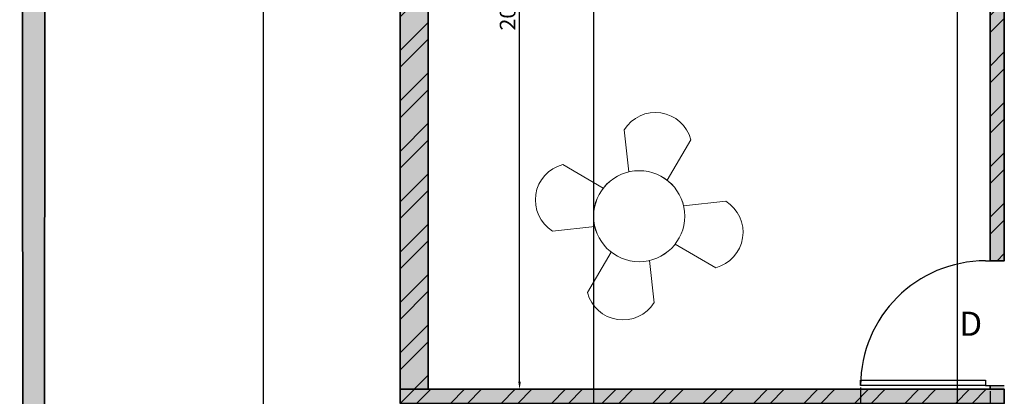
# Model space of a CAD drawing. Units: inches. Extents: x 1804 to 3296, y 909 to 2477.
# Tile 11 of 31: x 1804 to 2119, y 1542 to 1663. Entities that reach past the tile are written whole.
import ezdxf

# ---------------------------------------------------------------- set-up
doc = ezdxf.new("R2010")
doc.units = ezdxf.units.IN
for name, color, linetype, lineweight in [('A-ANNO-DIMS', 2, 'Continuous', 18), ('A-ANNO-TTLB', 156, 'Continuous', 35), ('A-WALL-PATT', 10, 'Continuous', 13), ('DOOR', 30, 'Continuous', 25), ('FUR', 100, 'Continuous', 18), ('TEXT', 190, 'Continuous', 18), ('WALL', 10, 'Continuous', 35)]:
    doc.layers.add(name, color=color, linetype=linetype, lineweight=lineweight)
doc.styles.get("Standard").update_dxf_attribs({"font": 'arial.ttf'})
doc.dimstyles.new('ISO-25', dxfattribs={"dimtxt": 5, "dimasz": 2.5, "dimexe": 1.25, "dimexo": 0.625, "dimtad": 1, "dimdec": 0, "dimlunit": 4, "dimtxsty": 'Standard', "dimcen": 2.5, "dimadec": 0, "dimazin": 0, "dimtfac": 1, "dimtdec": 0, "dimtmove": 0, "dimatfit": 3, "dimfxl": 1, "dimarcsym": 0})
pattern_1 = [(45, (0, 196.207), (-8.08223, 8.08223), []), (45, (5.388, 196.207), (-8.08223, 8.08223), [])]

# ---------------------------------------------------------------- blocks, each defined once
blk = doc.blocks.new('*U2')
for p, q in [((0, 0), (0, -6)), ((40, 0), (40, -6))]:
    blk.add_line(p, q)
blk.add_lwpolyline([(0, 0), (0, 40), (1.75, 40), (1.75, 0)], close=True)
blk.add_arc((0, 0), 40, 0, 90)
blk = doc.blocks.new('*U6')
for p, q in [((-4.25, 4.88), (-5.75, 18.4)), ((7.97, 2.19), (15.56, 15.17))]:
    blk.add_line(p, q)
blk.add_circle((-0.97, -9.34), 14.59)
blk.add_arc((4.21, 12.19), 11.73, 14.6829, 148.0797)
blk = doc.blocks.new('*U7')
at = {"layer": 'FUR', "transparency": 16777216}
blk.add_blockref('*U6', (1241.51, 881.82), dxfattribs=at)
for p, rotation in [((1231.21, 873.45), 89.99999999999999), ((1239.57, 863.15), 180), ((1249.88, 871.52), 269.9999999999999)]:
    blk.add_blockref('*U6', p, dxfattribs=dict(at, rotation=rotation))
blk = doc.blocks.new('*D9')
at = {"layer": 'A-ANNO-DIMS', "color": 0, "lineweight": -2, "transparency": 16777216}
for p, q in [((1935.21, 1793.38), (1965.1, 1793.38)), ((1963.85, 1546.88), (1963.85, 1790.88)), ((1935.21, 1544.38), (1965.1, 1544.38))]:
    blk.add_line(p, q, dxfattribs=at)
at = {"layer": 'A-ANNO-DIMS', "color": 0, "lineweight": 100, "transparency": 16777216}
for points in [[(1963.44, 1790.88), (1964.27, 1790.88), (1963.85, 1793.38)], [(1963.44, 1546.88), (1964.27, 1546.88), (1963.85, 1544.38)]]:
    blk.add_solid(points, dxfattribs=at)
at = {"layer": 'Defpoints', "color": 0, "lineweight": 100, "transparency": 16777216}
for p in [(1934.58, 1793.38), (1963.85, 1793.38), (1934.58, 1544.38)]:
    blk.add_point(p, dxfattribs=at)
at = {"layer": 'A-ANNO-DIMS', "color": 0, "transparency": 16777216, "insert": (1960.67, 1668.88), "char_height": 5, "attachment_point": 5, "rotation": 90}
blk.add_mtext('20\'-9"', dxfattribs=at)
blk = doc.blocks.new('*D52')
at = {"layer": 'A-ANNO-DIMS', "color": 0, "lineweight": -2, "transparency": 16777216}
for p, q in [((1924.96, 1830.04), (1880.63, 1830.04)), ((1881.88, 1065.27), (1881.88, 1827.54)), ((1924.96, 1062.77), (1880.63, 1062.77))]:
    blk.add_line(p, q, dxfattribs=at)
at = {"layer": 'A-ANNO-DIMS', "color": 0, "lineweight": 100, "transparency": 16777216}
for points in [[(1881.47, 1827.54), (1882.3, 1827.54), (1881.88, 1830.04)], [(1881.47, 1065.27), (1882.3, 1065.27), (1881.88, 1062.77)]]:
    blk.add_solid(points, dxfattribs=at)
at = {"layer": 'Defpoints', "color": 0, "lineweight": 100, "transparency": 16777216}
for p in [(1881.88, 1830.04), (1925.58, 1830.04), (1925.58, 1062.77)]:
    blk.add_point(p, dxfattribs=at)
at = {"layer": 'A-ANNO-DIMS', "color": 0, "transparency": 16777216, "insert": (1878.67, 1446.4), "char_height": 5, "attachment_point": 5, "rotation": 90}
blk.add_mtext('63\'-11 1/2"', dxfattribs=at)
blk = doc.blocks.new('*D60')
at = {"layer": 'A-ANNO-DIMS', "color": 0, "lineweight": -2, "transparency": 16777216}
for p, q in [((2073.08, 1544.95), (2073.08, 975.89)), ((2114.58, 1543.75), (2114.58, 975.89)), ((2112.08, 977.14), (2075.58, 977.14))]:
    blk.add_line(p, q, dxfattribs=at)
at = {"layer": 'A-ANNO-DIMS', "color": 0, "lineweight": 100, "transparency": 16777216}
for points in [[(2075.58, 977.56), (2075.58, 976.72), (2073.08, 977.14)], [(2112.08, 977.56), (2112.08, 976.72), (2114.58, 977.14)]]:
    blk.add_solid(points, dxfattribs=at)
at = {"layer": 'Defpoints', "color": 0, "lineweight": 100, "transparency": 16777216}
for p in [(2073.08, 1545.58), (2114.58, 1544.38), (2073.08, 977.14)]:
    blk.add_point(p, dxfattribs=at)
at = {"layer": 'A-ANNO-DIMS', "color": 0, "transparency": 16777216, "insert": (2093.83, 980.35), "char_height": 5, "attachment_point": 5}
blk.add_mtext('3\'-5 1/2"', dxfattribs=at)
blk = doc.blocks.new('*D62')
at = {"layer": 'A-ANNO-DIMS', "color": 0, "lineweight": -2, "transparency": 16777216}
for p, q in [((1987.63, 1501.57), (1987.63, 1874.99)), ((1990.13, 1873.74), (2101.57, 1873.74)), ((2104.07, 1501.57), (2104.07, 1874.99))]:
    blk.add_line(p, q, dxfattribs=at)
at = {"layer": 'A-ANNO-DIMS', "color": 0, "lineweight": 100, "transparency": 16777216}
for points in [[(1990.13, 1874.15), (1990.13, 1873.32), (1987.63, 1873.74)], [(2101.57, 1874.15), (2101.57, 1873.32), (2104.07, 1873.74)]]:
    blk.add_solid(points, dxfattribs=at)
at = {"layer": 'Defpoints', "color": 0, "lineweight": 100, "transparency": 16777216}
for p in [(2104.07, 1873.74), (1987.63, 1500.95), (2104.07, 1500.95)]:
    blk.add_point(p, dxfattribs=at)
at = {"layer": 'A-ANNO-DIMS', "color": 0, "transparency": 16777216, "insert": (2045.85, 1876.95), "char_height": 5, "attachment_point": 5}
blk.add_mtext('9\'-8 1/2"', dxfattribs=at)

msp = doc.modelspace()

# ---------------------------------------------------------------- hatches: boundary and pattern name
at = {"layer": 'A-ANNO-TTLB'}
h = msp.add_hatch(color=256, dxfattribs=at)
h.dxf.hatch_style = 1
h.paths.add_polyline_path([(3294.53, 2476.54), (1803.79, 2476.54), (1805.43, 909.47), (3296.17, 909.47)])
h.paths.add_polyline_path([(1811, 914.33), (1812.79, 2467.54), (3285.53, 2467.54), (3283.74, 914.33)], flags=16)
h.paths.add_polyline_path([(1925.58, 1062.77), (1925.58, 1138.07), (1925.58, 1539.88), (1925.58, 1793.38), (1925.58, 1830.04), (2325.54, 1830.04), (2325.54, 1793.38), (2325.54, 1586.42), (2325.54, 1138.07), (2325.54, 1062.77)], flags=0)
h.paths.add_polyline_path([(1997.22, 1029.4), (2008.85, 1037.96), (2008.85, 1020.84)], flags=0)
h.paths.add_polyline_path([(1934.58, 1138.07), (1934.58, 1147.07), (2078.77, 1147.07), (2078.77, 1138.07), (2060.94, 1138.07)], flags=0)
h.paths.add_polyline_path([(1944.35, 1138.07), (1944.35, 1147.07), (2056.05, 1147.07), (2056.05, 1138.07)], flags=0)
h.paths.add_polyline_path([(2222.24, 1037.96), (2233.87, 1029.4), (2222.24, 1020.84)], flags=0)
h.paths.add_polyline_path([(2061.94, 1139.07), (2061.94, 1146.07), (2077.77, 1146.07), (2077.77, 1139.07)], flags=0)
h.paths.add_polyline_path([(2149.58, 1138.07), (2149.58, 1269.44), (2158.58, 1269.44), (2158.58, 1326.69), (2149.58, 1326.69), (2149.58, 1340.94), (2139.6, 1340.94), (2139.6, 1434.25), (2149.58, 1434.25), (2149.58, 1447.36), (2158.58, 1447.36), (2158.58, 1423.87), (2158.58, 1408.06), (2198.46, 1408.06), (2198.46, 1412.56), (2282.65, 1412.56), (2282.65, 1465.94), (2316.54, 1465.94), (2316.54, 1590.92), (2192.86, 1590.92), (2192.86, 1595.3), (2291.17, 1595.3), (2291.17, 1590.92), (2316.54, 1590.92), (2316.54, 1784.38), (2300.24, 1784.38), (2300.24, 1757.47), (2268, 1757.47), (2268, 1681.04), (2180.87, 1681.04), (2180.87, 1757.47), (2148.63, 1757.47), (2148.63, 1784.38), (2119.08, 1784.38), (2119.08, 1585.58), (2114.58, 1585.58), (2114.58, 1784.38), (2064.11, 1784.38), (2046.28, 1784.38), (2046.28, 1760.38), (1958.58, 1760.38), (1958.58, 1664.38), (1934.58, 1664.38), (1934.58, 1784.38), (1934.58, 1793.38), (2046.28, 1793.38), (2064.11, 1793.38), (2119.08, 1793.38), (2230.78, 1793.38), (2230.78, 1784.38), (2268, 1784.38), (2300.24, 1784.38), (2316.54, 1784.38), (2316.54, 1590.92), (2316.54, 1373.73), (2316.54, 1138.07)], flags=0)
h.paths.add_polyline_path([(2209.19, 1166.63), (2209.19, 1175.63), (2158.58, 1175.63), (2209.19, 1223.63), (2209.19, 1231.63), (2183.88, 1231.63), (2183.88, 1301.66), (2242.59, 1301.66), (2242.59, 1326.69), (2316.54, 1326.69), (2272.59, 1271.63), (2272.59, 1223.63), (2316.54, 1175.63), (2272.59, 1175.63), (2272.59, 1166.63)], flags=0)
h.paths.add_polyline_path([(1947.77, 1345.22), (1947.77, 1457.48), (1991.2, 1457.48), (1991.2, 1451.7), (1991.2, 1352.18), (1991.2, 1345.22)], flags=0)
h.paths.add_polyline_path([(2209.19, 1271.63), (2262.59, 1271.63), (2262.59, 1311.85), (2272.59, 1301.66), (2272.59, 1271.63), (2269.92, 1269.63), (2270.59, 1269.63), (2270.59, 1225.63), (2211.19, 1225.63), (2211.19, 1269.63), (2211.86, 1269.63)], flags=0)
h.paths.add_polyline_path([(2000.34, 1378.21), (2000.34, 1429.71), (2025.22, 1429.71), (2025.22, 1378.21)], flags=0)
h.paths.add_polyline_path([(2001.34, 1379.21), (2001.34, 1428.71), (2024.22, 1428.71), (2024.22, 1379.21)], flags=0)
h.paths.add_polyline_path([(2012.34, 1390.21), (2012.34, 1417.71), (2013.22, 1417.71), (2013.22, 1390.21)], flags=0)
h.paths.add_polyline_path([(2237.56, 1331.19), (2237.56, 1340.18), (2238.62, 1340.18), (2238.62, 1386.84), (2241.04, 1386.84), (2242.06, 1386.84), (2242.06, 1408.06), (2316.54, 1331.19)], flags=0)
h.paths.add_polyline_path([(1953.73, 1464.35), (1953.73, 1498.59), (1981.74, 1498.59), (1981.74, 1464.35)], flags=0)
h.paths.add_polyline_path([(1987.63, 1462.08), (1987.63, 1500.95), (2104.07, 1500.95), (2104.07, 1462.08), (2099.27, 1462.08), (1993.6, 1462.08)], flags=0)
h.paths.add_polyline_path([(1956.06, 1481.47, -1), (1979.41, 1481.47, -1)], flags=0)
edge = h.paths.add_edge_path(flags=0)
edge.add_ellipse((2299.53, 1438.37), major_axis=(0.31, 21.36), ratio=0.670333, start_angle=0, end_angle=360)
h.paths.add_polyline_path([(2297.39, 1438.37, -1), (2301.67, 1438.37, -1)], flags=0)
h.paths.add_polyline_path([(2591.54, 1163.23), (2591.54, 1179.38), (2591.54, 1379.68), (2591.54, 1395.84), (2734.5, 1395.84), (2734.5, 1379.68), (2734.5, 1179.38), (2734.5, 1163.23)], flags=0)
h.paths.add_polyline_path([(2592.54, 1164.23), (2592.54, 1166.23), (2733.5, 1166.23), (2733.5, 1164.23)], flags=0)
h.paths.add_polyline_path([(2592.54, 1180.38), (2592.54, 1378.68), (2733.5, 1378.68), (2733.5, 1180.38)], flags=0)
h.paths.add_polyline_path([(2593.54, 1181.38), (2593.54, 1377.68), (2732.5, 1377.68), (2732.5, 1181.38)], flags=0)
h.paths.add_polyline_path([(2594.54, 1182.38), (2594.54, 1376.68), (2731.5, 1376.68), (2731.5, 1182.38)], flags=0)
h.paths.add_polyline_path([(1936.95, 1697.46), (1936.95, 1736.46), (1955.41, 1736.46), (1955.41, 1697.46)], flags=0)
h.paths.add_polyline_path([(1938.48, 1718.36), (1938.48, 1734.92), (1953.65, 1734.92), (1953.65, 1718.36)], flags=0)
h.paths.add_polyline_path([(1944.75, 1726.64, -1), (1947.37, 1726.64, -1)], flags=0)
h.paths.add_polyline_path([(2592.54, 1394.84), (2733.5, 1394.84), (2733.5, 1392.84), (2592.54, 1392.84)], flags=0)
h.paths.add_polyline_path([(1976.61, 1762.5), (1976.61, 1781.44), (2012.79, 1781.44), (2012.79, 1762.5)], flags=0)
h.paths.add_polyline_path([(1979.57, 1771.97, -1), (1991.39, 1771.97, -1)], flags=0)
h.paths.add_polyline_path([(1995.36, 1771.97, -1), (2007.18, 1771.97, -1)], flags=0)
h.paths.add_polyline_path([(2251.51, 1744.53), (2268, 1730.05), (2251.51, 1730.05)], flags=0)
h.paths.add_polyline_path([(2047.28, 1785.38), (2047.28, 1792.38), (2063.11, 1792.38), (2063.11, 1785.38)], flags=0)
h.paths.add_polyline_path([(2155.08, 1770.92, -1), (2174.42, 1770.92, -1)], flags=0)
h.paths.add_polyline_path([(2188.59, 1758.27), (2188.59, 1772.81), (2222.3, 1772.81), (2222.3, 1758.27)], flags=0)
h.paths.add_polyline_path([(2223.97, 1758.27), (2223.97, 1772.81), (2257.68, 1772.81), (2257.68, 1758.27)], flags=0)
h.paths.add_polyline_path([(2274.45, 1770.92, -1), (2293.8, 1770.92, -1)], flags=0)
h.paths.add_polyline_path([(2591.54, 1582.09), (2591.54, 1782.39), (2734.5, 1782.39), (2734.5, 1582.09)], flags=0)
h.paths.add_polyline_path([(2592.54, 1583.09), (2592.54, 1781.39), (2733.5, 1781.39), (2733.5, 1583.09)], flags=0)
h.paths.add_polyline_path([(2593.54, 1584.09), (2593.54, 1780.39), (2732.5, 1780.39), (2732.5, 1584.09)], flags=0)
h.paths.add_polyline_path([(2594.54, 1585.09), (2594.54, 1779.39), (2731.5, 1779.39), (2731.5, 1585.09)], flags=0)
h.paths.add_polyline_path([(1922.17, 1978.79), (1922.17, 2295.08), (1922.17, 2296.08), (2115.67, 2296.08), (2115.67, 2384.31), (2115.67, 2385.31), (2322.12, 2385.31), (2323.12, 2385.31), (2323.12, 1979.79), (2323.12, 1978.79), (1923.17, 1978.79)], flags=0)
h.paths.add_polyline_path([(1922.17, 1978.79), (1922.17, 2051.31), (1922.17, 2214.86), (1922.17, 2296.08), (2115.67, 2296.08), (2115.67, 2385.31), (2323.12, 2385.31), (2323.12, 2280.42), (2323.12, 1978.79), (2115.67, 1978.79)], flags=0)
h.paths.add_polyline_path([(1923.17, 1979.79), (1923.17, 2050.31), (2115.67, 2050.31), (2115.67, 2051.31), (1923.17, 2051.31), (1923.17, 2213.86), (1923.17, 2214.86), (1923.17, 2295.08), (1990.02, 2295.08), (1990.02, 2214.86), (1991.02, 2214.86), (1991.02, 2295.08), (2115.67, 2295.08), (2115.67, 1979.79), (2116.67, 1979.79), (2116.67, 2304.18), (2116.67, 2384.31), (2322.12, 2384.31), (2322.12, 2280.42), (2322.12, 1979.79), (2115.67, 1979.79)], flags=0)
h.paths.add_polyline_path([(2972.46, 1192.5), (2972.46, 1196.92), (2995.47, 1196.92), (2995.47, 1255.47), (2995.09, 1255.47), (2987.42, 1249.39), (2980.08, 1255.47), (2978.05, 1255.47), (2978.05, 1257.24), (2995.47, 1257.24), (2995.47, 1261.58), (3015.37, 1261.58), (3015.37, 1333.28), (3015.37, 1414.4), (3032.82, 1414.4), (3032.82, 1333.28), (3032.82, 1261.58), (3052.66, 1261.58), (3052.66, 1255.47), (3079.86, 1255.47), (3078.72, 1254.57), (3081.47, 1252.29), (3078.56, 1249.99), (3075.81, 1252.26), (3072.57, 1249.69), (3070.36, 1251.52), (3067.67, 1249.39), (3060.34, 1255.47), (3052.66, 1255.47), (3052.66, 1196.92), (3054.58, 1196.92), (3074, 1196.92), (3074, 1192.5), (3052.66, 1192.5), (2995.47, 1192.5)], flags=0)
h.paths.add_polyline_path([(2490.75, 1979.27), (2490.75, 1980.27), (2596.87, 1980.27), (2596.87, 2051.8), (2596.87, 2052.8), (2596.87, 2216.35), (2596.87, 2297.57), (2717.32, 2297.57), (2710.57, 2305.62), (2724.07, 2305.62), (2717.32, 2297.57), (2782.37, 2297.57), (2782.37, 2395.8), (3006.82, 2395.8), (3006.82, 1981.27), (3093.73, 1981.27), (3093.73, 1980.27), (3047.51, 1980.27), (3046.37, 1979.37), (3049.11, 1977.1), (3046.2, 1974.79), (3043.46, 1977.07), (3040.21, 1974.49), (3038, 1976.32), (3035.32, 1974.2), (3027.98, 1980.27), (2871.83, 1980.27), (2871.83, 1981.27), (2791.37, 1981.27), (2791.37, 2050.8), (2597.87, 2050.8), (2597.87, 1980.27), (2597.87, 1979.27), (2546.27, 1979.27), (2545.12, 1978.37), (2547.87, 1976.1), (2544.96, 1973.79), (2542.22, 1976.07), (2538.97, 1973.49), (2536.76, 1975.32), (2534.07, 1973.2), (2526.74, 1979.27)], flags=0)
h.paths.add_polyline_path([(2597.87, 2051.8), (2606.87, 2051.8), (2606.87, 2258.39), (2597.87, 2258.39), (2597.87, 2296.57), (2606.87, 2296.57), (2606.87, 2262.39), (2782.37, 2262.39), (2782.37, 2296.57), (2790.37, 2296.57), (2790.37, 2262.39), (2791.37, 2262.39), (2791.37, 2305.67), (2791.37, 2385.8), (2996.82, 2385.8), (2996.82, 2339.85), (3006.82, 2339.85), (3006.82, 2250.12), (2997.82, 2250.12), (2997.82, 1981.27), (2996.82, 1981.27), (2872.83, 1981.27), (2872.83, 1991.8), (2871.83, 1991.8), (2871.83, 2050.8), (2790.37, 2050.8), (2597.87, 2050.8)], flags=0)
h.paths.add_polyline_path([(2179.93, 2153.92), (2179.93, 2353.97), (2259.98, 2353.97), (2259.98, 2153.92)], flags=0)
h.paths.add_polyline_path([(2180.93, 2154.92), (2180.93, 2352.97), (2258.98, 2352.97), (2258.98, 2154.92)], flags=0)
h.paths.add_polyline_path([(2960.87, 1608.49), (2960.87, 1753.62), (3070.9, 1753.62), (3070.9, 1608.49)], flags=0)
h.paths.add_polyline_path([(2961.87, 1609.49), (2961.87, 1752.62), (3069.9, 1752.62), (3069.9, 1609.49)], flags=0)
h.paths.add_polyline_path([(2962.87, 1610.49), (2962.87, 1751.62), (3068.9, 1751.62), (3068.9, 1610.49)], flags=0)
h.paths.add_polyline_path([(2963.87, 1611.49), (2963.87, 1750.62), (3067.9, 1750.62), (3067.9, 1611.49)], flags=0)
h.paths.add_polyline_path([(2782.37, 2051.8), (2782.37, 2216.32), (2791.37, 2216.32), (2791.37, 2051.8), (2872.83, 2051.8), (2872.83, 2068.56), (2884.67, 2068.56), (2884.67, 2085.33), (2896.51, 2085.33), (2896.51, 2102.09), (2908.36, 2102.09), (2908.36, 2118.85), (2920.2, 2118.85), (2920.2, 2135.62), (2932.05, 2135.62), (2932.05, 2145.3), (2925.08, 2145.3), (2925.08, 2203.2), (2996.82, 2203.2), (2996.82, 2145.3), (2953.82, 2145.3), (2872.83, 2051.8), (2790.37, 2051.8)], flags=0)
h.paths.add_polyline_path([(2717.32, 2238.65), (2710.57, 2246.7), (2724.07, 2246.7)], flags=0)
h.paths.add_polyline_path([(2003.09, 1122.79), (2017.16, 1122.79), (2017.16, 1138.74), (2003.09, 1138.74)], flags=8)
h.paths.add_polyline_path([(2174.76, 1792.72), (2188.83, 1792.72), (2188.83, 1808.66), (2174.76, 1808.66)], flags=8)
h.paths.add_polyline_path([(1987.95, 1792.51), (2002.02, 1792.51), (2002.02, 1808.45), (1987.95, 1808.45)], flags=8)
h.paths.add_polyline_path([(2148.79, 1289.26), (2160.46, 1289.26), (2160.46, 1305.2), (2148.79, 1305.2)], flags=8)
h.paths.add_polyline_path([(2115.36, 1133.57), (2127.04, 1133.57), (2127.04, 1149.51), (2115.36, 1149.51)], flags=8)
h.paths.add_polyline_path([(2237.58, 1421.48), (2249.25, 1421.48), (2249.25, 1437.43), (2237.58, 1437.43)], flags=8)
h.paths.add_polyline_path([(2134.99, 1584.32), (2146.66, 1584.32), (2146.66, 1600.26), (2134.99, 1600.26)], flags=8)
h.paths.add_polyline_path([(2101.95, 1557.31), (2113.62, 1557.31), (2113.62, 1573.25), (2101.95, 1573.25)], flags=8)
h.paths.add_polyline_path([(2937.85, 1156.77), (3120.41, 1156.77), (3120.41, 1185.72), (2937.85, 1185.72)], flags=8)
h.paths.add_polyline_path([(2980.71, 1786.71), (3050.06, 1786.71), (3050.06, 1802.66), (2980.71, 1802.66)], flags=8)
h.paths.add_polyline_path([(2869.28, 1661.96), (2938.62, 1661.96), (2938.62, 1690.8), (2869.28, 1690.8)], flags=8)
h.paths.add_polyline_path([(3092.27, 1674.86), (3161.62, 1674.86), (3161.62, 1690.8), (3092.27, 1690.8)], flags=8)
h.paths.add_polyline_path([(2980.71, 1674.86), (3050.06, 1674.86), (3050.06, 1690.8), (2980.71, 1690.8)], flags=8)
h.paths.add_polyline_path([(2649.07, 1678.23), (2674.53, 1678.23), (2674.53, 1714.76), (2649.07, 1714.76)], flags=8)
h.paths.add_polyline_path([(2530.84, 1981.63), (2549.13, 1981.63), (2549.13, 1997.57), (2530.84, 1997.57)], flags=8)
h.paths.add_polyline_path([(3031.29, 1981.77), (3049.58, 1981.77), (3049.58, 1997.71), (3031.29, 1997.71)], flags=8)
h.paths.add_polyline_path([(2715.38, 1911.9), (2851.54, 1911.9), (2851.54, 1940.85), (2715.38, 1940.85)], flags=8)
h.paths.add_polyline_path([(2015.23, 1927.36), (2205.42, 1927.36), (2205.42, 1956.3), (2015.23, 1956.3)], flags=8)
h.paths.add_polyline_path([(2671.84, 2057.84), (2702.75, 2057.84), (2702.75, 2073.79), (2671.84, 2073.79)], flags=8)
h.paths.add_polyline_path([(2678.5, 2316.52), (2765.26, 2316.52), (2765.26, 2332.46), (2678.5, 2332.46)], flags=8)
h.paths.add_polyline_path([(2678.48, 2271.96), (2736.41, 2271.96), (2736.41, 2287.9), (2678.48, 2287.9)], flags=8)
h.paths.add_polyline_path([(2019.2, 972.79), (2243.21, 972.79), (2243.21, 1001.74), (2019.2, 1001.74)], flags=8)
h.paths.add_polyline_path([(2097.06, 1021.56), (2132.16, 1021.56), (2132.16, 1037.51), (2097.06, 1037.51)], flags=8)
h.paths.add_polyline_path([(2182.47, 1360.48), (2207.35, 1360.48), (2207.35, 1376.42), (2182.47, 1376.42)], flags=8)
h.paths.add_polyline_path([(2261.12, 1361.77), (2295.01, 1361.77), (2295.01, 1377.71), (2261.12, 1377.71)], flags=8)
h.paths.add_polyline_path([(2245.75, 1511.51), (2278.44, 1511.51), (2278.44, 1527.46), (2245.75, 1527.46)], flags=8)
h.paths.add_polyline_path([(1991.16, 1296.29), (2060.51, 1296.29), (2060.51, 1312.23), (1991.16, 1312.23)], flags=8)
h.paths.add_polyline_path([(2187, 1651.35), (2246.71, 1651.35), (2246.71, 1667.29), (2187, 1667.29)], flags=8)
h.paths.add_polyline_path([(1976.49, 1684.81), (2068.63, 1684.81), (2068.63, 1700.76), (1976.49, 1700.76)], flags=8)
at = {"layer": 'A-WALL-PATT'}
h = msp.add_hatch(color=256, dxfattribs=at)
h.dxf.hatch_style = 1
h.paths.add_polyline_path([(2119.08, 1544.38), (1925.58, 1544.38), (1925.58, 1539.88), (2119.08, 1539.88)])
h.paths.add_polyline_path([(2119.08, 1545.58), (2114.58, 1545.58), (2114.58, 1544.38), (2119.08, 1544.38)])
h.paths.add_polyline_path([(1965.87, 1658.79), (1965.87, 1679.09), (1955.57, 1679.09), (1955.57, 1658.79)], flags=9)
h.paths.add_polyline_path([(2293.18, 1677.29), (2293.18, 1697.58), (2282.88, 1697.58), (2282.88, 1677.29)], flags=9)
h.paths.add_polyline_path([(2271.13, 1545.23), (2287.53, 1545.23), (2287.53, 1555.53), (2271.13, 1555.53)], flags=9)
h.paths.add_polyline_path([(2303.26, 1488.52), (2303.26, 1508.82), (2292.95, 1508.82), (2292.95, 1488.52)], flags=9)
h.paths.add_polyline_path([(2271.13, 1393.15), (2287.53, 1393.15), (2287.53, 1403.45), (2271.13, 1403.45)], flags=9)
h.paths.add_polyline_path([(2306.48, 1361.45), (2306.48, 1377.86), (2296.18, 1377.86), (2296.18, 1361.45)], flags=9)
h.paths.add_polyline_path([(2174.54, 1361.45), (2174.54, 1377.86), (2164.23, 1377.86), (2164.23, 1361.45)], flags=9)
h.paths.add_polyline_path([(1968.21, 1333.34), (1968.21, 1353.64), (1957.91, 1353.64), (1957.91, 1333.34)], flags=9)
h.paths.add_polyline_path([(2003.09, 1122.79), (2017.16, 1122.79), (2017.16, 1138.74), (2003.09, 1138.74)], flags=9)
h.paths.add_polyline_path([(2174.76, 1792.72), (2188.83, 1792.72), (2188.83, 1808.66), (2174.76, 1808.66)], flags=9)
h.paths.add_polyline_path([(1987.95, 1792.51), (2002.02, 1792.51), (2002.02, 1808.45), (1987.95, 1808.45)], flags=9)
h.paths.add_polyline_path([(2148.79, 1289.26), (2160.46, 1289.26), (2160.46, 1305.2), (2148.79, 1305.2)], flags=9)
h.paths.add_polyline_path([(2115.36, 1133.57), (2127.04, 1133.57), (2127.04, 1149.51), (2115.36, 1149.51)], flags=9)
h.paths.add_polyline_path([(2237.58, 1421.48), (2249.25, 1421.48), (2249.25, 1437.43), (2237.58, 1437.43)], flags=9)
h.paths.add_polyline_path([(2134.99, 1584.32), (2146.66, 1584.32), (2146.66, 1600.26), (2134.99, 1600.26)], flags=9)
h.paths.add_polyline_path([(2101.95, 1557.31), (2113.62, 1557.31), (2113.62, 1573.25), (2101.95, 1573.25)], flags=9)
h.paths.add_polyline_path([(2937.85, 1156.77), (3120.41, 1156.77), (3120.41, 1185.72), (2937.85, 1185.72)], flags=9)
h.paths.add_polyline_path([(2980.71, 1786.71), (3050.06, 1786.71), (3050.06, 1802.66), (2980.71, 1802.66)], flags=9)
h.paths.add_polyline_path([(2869.28, 1661.96), (2938.62, 1661.96), (2938.62, 1690.8), (2869.28, 1690.8)], flags=9)
h.paths.add_polyline_path([(3092.27, 1674.86), (3161.62, 1674.86), (3161.62, 1690.8), (3092.27, 1690.8)], flags=9)
h.paths.add_polyline_path([(2980.71, 1674.86), (3050.06, 1674.86), (3050.06, 1690.8), (2980.71, 1690.8)], flags=9)
h.paths.add_polyline_path([(2649.07, 1678.23), (2674.53, 1678.23), (2674.53, 1714.76), (2649.07, 1714.76)], flags=9)
h.paths.add_polyline_path([(2530.84, 1981.63), (2549.13, 1981.63), (2549.13, 1997.57), (2530.84, 1997.57)], flags=9)
h.paths.add_polyline_path([(3031.29, 1981.77), (3049.58, 1981.77), (3049.58, 1997.71), (3031.29, 1997.71)], flags=9)
h.paths.add_polyline_path([(2715.38, 1911.9), (2851.54, 1911.9), (2851.54, 1940.85), (2715.38, 1940.85)], flags=9)
h.paths.add_polyline_path([(2015.23, 1927.36), (2205.42, 1927.36), (2205.42, 1956.3), (2015.23, 1956.3)], flags=9)
h.paths.add_polyline_path([(2671.84, 2057.84), (2702.75, 2057.84), (2702.75, 2073.79), (2671.84, 2073.79)], flags=9)
h.paths.add_polyline_path([(2678.5, 2316.52), (2765.26, 2316.52), (2765.26, 2332.46), (2678.5, 2332.46)], flags=9)
h.paths.add_polyline_path([(2678.48, 2271.96), (2736.41, 2271.96), (2736.41, 2287.9), (2678.48, 2287.9)], flags=9)
h.paths.add_polyline_path([(2019.2, 972.79), (2243.21, 972.79), (2243.21, 1001.74), (2019.2, 1001.74)], flags=9)
h.paths.add_polyline_path([(2097.06, 1021.56), (2132.16, 1021.56), (2132.16, 1037.51), (2097.06, 1037.51)], flags=9)
h.paths.add_polyline_path([(2182.47, 1360.48), (2207.35, 1360.48), (2207.35, 1376.42), (2182.47, 1376.42)], flags=9)
h.paths.add_polyline_path([(2261.12, 1361.77), (2295.01, 1361.77), (2295.01, 1377.71), (2261.12, 1377.71)], flags=9)
h.paths.add_polyline_path([(2245.75, 1511.51), (2278.44, 1511.51), (2278.44, 1527.46), (2245.75, 1527.46)], flags=9)
h.paths.add_polyline_path([(1991.16, 1296.29), (2060.51, 1296.29), (2060.51, 1312.23), (1991.16, 1312.23)], flags=9)
h.paths.add_polyline_path([(2187, 1651.35), (2246.71, 1651.35), (2246.71, 1667.29), (2187, 1667.29)], flags=9)
h.paths.add_polyline_path([(1976.49, 1684.81), (2068.63, 1684.81), (2068.63, 1700.76), (1976.49, 1700.76)], flags=9)
h = msp.add_hatch(color=256, dxfattribs=at)
h.dxf.hatch_style = 1
h.paths.add_polyline_path([(2149.58, 1147.07), (2141.21, 1147.07), (2141.21, 1144.07), (2141.21, 1138.07), (2149.58, 1138.07)])
h.paths.add_polyline_path([(2101.21, 1144.07, -0.01877), (2101.32, 1147.07), (2078.77, 1147.07), (2078.77, 1138.07), (2101.21, 1138.07)])
h.paths.add_polyline_path([(2060.94, 1147.07), (2056.05, 1147.07), (2056.05, 1138.07), (2060.94, 1138.07)])
h.paths.add_polyline_path([(1944.35, 1147.07), (1934.58, 1147.07), (1934.58, 1138.07), (1944.35, 1138.07)])
h.paths.add_polyline_path([(2158.58, 1269.44), (2149.58, 1269.44), (2149.58, 1138.07), (2158.58, 1138.07)])
h.paths.add_polyline_path([(2003.09, 1122.79), (2017.16, 1122.79), (2017.16, 1138.74), (2003.09, 1138.74)], flags=9)
h.paths.add_polyline_path([(2174.76, 1792.72), (2188.83, 1792.72), (2188.83, 1808.66), (2174.76, 1808.66)], flags=9)
h.paths.add_polyline_path([(1987.95, 1792.51), (2002.02, 1792.51), (2002.02, 1808.45), (1987.95, 1808.45)], flags=9)
h.paths.add_polyline_path([(2148.79, 1289.26), (2160.46, 1289.26), (2160.46, 1305.2), (2148.79, 1305.2)], flags=9)
h.paths.add_polyline_path([(2115.36, 1133.57), (2127.04, 1133.57), (2127.04, 1149.51), (2115.36, 1149.51)], flags=9)
h.paths.add_polyline_path([(2237.58, 1421.48), (2249.25, 1421.48), (2249.25, 1437.43), (2237.58, 1437.43)], flags=9)
h.paths.add_polyline_path([(2134.99, 1584.32), (2146.66, 1584.32), (2146.66, 1600.26), (2134.99, 1600.26)], flags=9)
h.paths.add_polyline_path([(2101.95, 1557.31), (2113.62, 1557.31), (2113.62, 1573.25), (2101.95, 1573.25)], flags=9)
h.paths.add_polyline_path([(2937.85, 1156.77), (3120.41, 1156.77), (3120.41, 1185.72), (2937.85, 1185.72)], flags=9)
h.paths.add_polyline_path([(2980.71, 1786.71), (3050.06, 1786.71), (3050.06, 1802.66), (2980.71, 1802.66)], flags=9)
h.paths.add_polyline_path([(2869.28, 1661.96), (2938.62, 1661.96), (2938.62, 1690.8), (2869.28, 1690.8)], flags=9)
h.paths.add_polyline_path([(3092.27, 1674.86), (3161.62, 1674.86), (3161.62, 1690.8), (3092.27, 1690.8)], flags=9)
h.paths.add_polyline_path([(2980.71, 1674.86), (3050.06, 1674.86), (3050.06, 1690.8), (2980.71, 1690.8)], flags=9)
h.paths.add_polyline_path([(2649.07, 1678.23), (2674.53, 1678.23), (2674.53, 1714.76), (2649.07, 1714.76)], flags=9)
h.paths.add_polyline_path([(2530.84, 1981.63), (2549.13, 1981.63), (2549.13, 1997.57), (2530.84, 1997.57)], flags=9)
h.paths.add_polyline_path([(3031.29, 1981.77), (3049.58, 1981.77), (3049.58, 1997.71), (3031.29, 1997.71)], flags=9)
h.paths.add_polyline_path([(2715.38, 1911.9), (2851.54, 1911.9), (2851.54, 1940.85), (2715.38, 1940.85)], flags=9)
h.paths.add_polyline_path([(2015.23, 1927.36), (2205.42, 1927.36), (2205.42, 1956.3), (2015.23, 1956.3)], flags=9)
h.paths.add_polyline_path([(2671.84, 2057.84), (2702.75, 2057.84), (2702.75, 2073.79), (2671.84, 2073.79)], flags=9)
h.paths.add_polyline_path([(2678.5, 2316.52), (2765.26, 2316.52), (2765.26, 2332.46), (2678.5, 2332.46)], flags=9)
h.paths.add_polyline_path([(2678.48, 2271.96), (2736.41, 2271.96), (2736.41, 2287.9), (2678.48, 2287.9)], flags=9)
h.paths.add_polyline_path([(2019.2, 972.79), (2243.21, 972.79), (2243.21, 1001.74), (2019.2, 1001.74)], flags=9)
h.paths.add_polyline_path([(2097.06, 1021.56), (2132.16, 1021.56), (2132.16, 1037.51), (2097.06, 1037.51)], flags=9)
h.paths.add_polyline_path([(2182.47, 1360.48), (2207.35, 1360.48), (2207.35, 1376.42), (2182.47, 1376.42)], flags=9)
h.paths.add_polyline_path([(2261.12, 1361.77), (2295.01, 1361.77), (2295.01, 1377.71), (2261.12, 1377.71)], flags=9)
h.paths.add_polyline_path([(2245.75, 1511.51), (2278.44, 1511.51), (2278.44, 1527.46), (2245.75, 1527.46)], flags=9)
h.paths.add_polyline_path([(1991.16, 1296.29), (2060.51, 1296.29), (2060.51, 1312.23), (1991.16, 1312.23)], flags=9)
h.paths.add_polyline_path([(2187, 1651.35), (2246.71, 1651.35), (2246.71, 1667.29), (2187, 1667.29)], flags=9)
h.paths.add_polyline_path([(1976.49, 1684.81), (2068.63, 1684.81), (2068.63, 1700.76), (1976.49, 1700.76)], flags=9)
h = msp.add_hatch(color=256, dxfattribs=at)
h.dxf.hatch_style = 1
h.paths.add_polyline_path([(2158.58, 1275.49), (2155.29, 1275.49), (2149.58, 1275.49), (2149.58, 1269.44), (2158.58, 1269.44)])
h.paths.add_polyline_path([(2158.58, 1326.69), (2149.58, 1326.69), (2149.58, 1319.33), (2155.29, 1319.33), (2158.58, 1319.33)])
h.paths.add_polyline_path([(2158.58, 1402.2), (2158.58, 1423.87), (2158.58, 1447.36), (2149.58, 1447.36), (2149.58, 1423.87), (2149.58, 1340.94), (2149.58, 1326.69), (2158.58, 1326.69), (2158.58, 1354.23)])
h.paths.add_polyline_path([(1965.87, 1658.79), (1965.87, 1679.09), (1955.57, 1679.09), (1955.57, 1658.79)], flags=9)
h.paths.add_polyline_path([(2293.18, 1677.29), (2293.18, 1697.58), (2282.88, 1697.58), (2282.88, 1677.29)], flags=9)
h.paths.add_polyline_path([(2271.13, 1545.23), (2287.53, 1545.23), (2287.53, 1555.53), (2271.13, 1555.53)], flags=9)
h.paths.add_polyline_path([(2303.26, 1488.52), (2303.26, 1508.82), (2292.95, 1508.82), (2292.95, 1488.52)], flags=9)
h.paths.add_polyline_path([(2271.13, 1393.15), (2287.53, 1393.15), (2287.53, 1403.45), (2271.13, 1403.45)], flags=9)
h.paths.add_polyline_path([(2306.48, 1361.45), (2306.48, 1377.86), (2296.18, 1377.86), (2296.18, 1361.45)], flags=9)
h.paths.add_polyline_path([(2189.9, 1340.62), (2206.31, 1340.62), (2206.31, 1350.92), (2189.9, 1350.92)], flags=9)
h.paths.add_polyline_path([(2174.54, 1361.45), (2174.54, 1377.86), (2164.23, 1377.86), (2164.23, 1361.45)], flags=9)
h.paths.add_polyline_path([(2304.24, 1240.8), (2304.24, 1261.09), (2293.94, 1261.09), (2293.94, 1240.8)], flags=9)
h.paths.add_polyline_path([(2227.19, 1188.73), (2247.49, 1188.73), (2247.49, 1199.03), (2227.19, 1199.03)], flags=9)
h.paths.add_polyline_path([(2181.93, 1144.21), (2181.93, 1160.62), (2171.63, 1160.62), (2171.63, 1144.21)], flags=9)
h.paths.add_polyline_path([(1968.21, 1333.34), (1968.21, 1353.64), (1957.91, 1353.64), (1957.91, 1333.34)], flags=9)
h.paths.add_polyline_path([(2029.78, 1203.53), (2053.95, 1203.53), (2053.95, 1213.83), (2029.78, 1213.83)], flags=9)
h.paths.add_polyline_path([(2576.51, 1671.88), (2576.51, 1692.17), (2566.21, 1692.17), (2566.21, 1671.88)], flags=9)
h.paths.add_polyline_path([(2566.99, 1269.67), (2566.99, 1289.96), (2556.68, 1289.96), (2556.68, 1269.67)], flags=9)
h.paths.add_polyline_path([(2581.85, 1269.17), (2581.85, 1289.46), (2571.54, 1289.46), (2571.54, 1269.17)], flags=9)
h.paths.add_polyline_path([(2650.71, 1409.75), (2674.89, 1409.75), (2674.89, 1420.05), (2650.71, 1420.05)], flags=9)
h.paths.add_polyline_path([(2003.09, 1122.79), (2017.16, 1122.79), (2017.16, 1138.74), (2003.09, 1138.74)], flags=9)
h.paths.add_polyline_path([(2174.76, 1792.72), (2188.83, 1792.72), (2188.83, 1808.66), (2174.76, 1808.66)], flags=9)
h.paths.add_polyline_path([(1987.95, 1792.51), (2002.02, 1792.51), (2002.02, 1808.45), (1987.95, 1808.45)], flags=9)
h.paths.add_polyline_path([(2148.79, 1289.26), (2160.46, 1289.26), (2160.46, 1305.2), (2148.79, 1305.2)], flags=9)
h.paths.add_polyline_path([(2115.36, 1133.57), (2127.04, 1133.57), (2127.04, 1149.51), (2115.36, 1149.51)], flags=9)
h.paths.add_polyline_path([(2237.58, 1421.48), (2249.25, 1421.48), (2249.25, 1437.43), (2237.58, 1437.43)], flags=9)
h.paths.add_polyline_path([(2134.99, 1584.32), (2146.66, 1584.32), (2146.66, 1600.26), (2134.99, 1600.26)], flags=9)
h.paths.add_polyline_path([(2101.95, 1557.31), (2113.62, 1557.31), (2113.62, 1573.25), (2101.95, 1573.25)], flags=9)
h.paths.add_polyline_path([(2937.85, 1156.77), (3120.41, 1156.77), (3120.41, 1185.72), (2937.85, 1185.72)], flags=9)
h.paths.add_polyline_path([(2980.71, 1786.71), (3050.06, 1786.71), (3050.06, 1802.66), (2980.71, 1802.66)], flags=9)
h.paths.add_polyline_path([(2869.28, 1661.96), (2938.62, 1661.96), (2938.62, 1690.8), (2869.28, 1690.8)], flags=9)
h.paths.add_polyline_path([(3092.27, 1674.86), (3161.62, 1674.86), (3161.62, 1690.8), (3092.27, 1690.8)], flags=9)
h.paths.add_polyline_path([(2980.71, 1674.86), (3050.06, 1674.86), (3050.06, 1690.8), (2980.71, 1690.8)], flags=9)
h.paths.add_polyline_path([(2649.07, 1678.23), (2674.53, 1678.23), (2674.53, 1714.76), (2649.07, 1714.76)], flags=9)
h.paths.add_polyline_path([(2530.84, 1981.63), (2549.13, 1981.63), (2549.13, 1997.57), (2530.84, 1997.57)], flags=9)
h.paths.add_polyline_path([(3031.29, 1981.77), (3049.58, 1981.77), (3049.58, 1997.71), (3031.29, 1997.71)], flags=9)
h.paths.add_polyline_path([(2715.38, 1911.9), (2851.54, 1911.9), (2851.54, 1940.85), (2715.38, 1940.85)], flags=9)
h.paths.add_polyline_path([(2015.23, 1927.36), (2205.42, 1927.36), (2205.42, 1956.3), (2015.23, 1956.3)], flags=9)
h.paths.add_polyline_path([(2671.84, 2057.84), (2702.75, 2057.84), (2702.75, 2073.79), (2671.84, 2073.79)], flags=9)
h.paths.add_polyline_path([(2678.5, 2316.52), (2765.26, 2316.52), (2765.26, 2332.46), (2678.5, 2332.46)], flags=9)
h.paths.add_polyline_path([(2678.48, 2271.96), (2736.41, 2271.96), (2736.41, 2287.9), (2678.48, 2287.9)], flags=9)
h.paths.add_polyline_path([(2019.2, 972.79), (2243.21, 972.79), (2243.21, 1001.74), (2019.2, 1001.74)], flags=9)
h.paths.add_polyline_path([(2097.06, 1021.56), (2132.16, 1021.56), (2132.16, 1037.51), (2097.06, 1037.51)], flags=9)
h.paths.add_polyline_path([(2182.47, 1360.48), (2207.35, 1360.48), (2207.35, 1376.42), (2182.47, 1376.42)], flags=9)
h.paths.add_polyline_path([(2261.12, 1361.77), (2295.01, 1361.77), (2295.01, 1377.71), (2261.12, 1377.71)], flags=9)
h.paths.add_polyline_path([(2245.75, 1511.51), (2278.44, 1511.51), (2278.44, 1527.46), (2245.75, 1527.46)], flags=9)
h.paths.add_polyline_path([(1991.16, 1296.29), (2060.51, 1296.29), (2060.51, 1312.23), (1991.16, 1312.23)], flags=9)
h.paths.add_polyline_path([(2187, 1651.35), (2246.71, 1651.35), (2246.71, 1667.29), (2187, 1667.29)], flags=9)
h.paths.add_polyline_path([(1976.49, 1684.81), (2068.63, 1684.81), (2068.63, 1700.76), (1976.49, 1700.76)], flags=9)
h = msp.add_hatch(dxfattribs=at)
h.set_pattern_fill('ANSI32', color=256, scale=1.2)
h.set_pattern_definition(pattern_1)
h.paths.add_polyline_path([(1934.58, 1784.38), (1934.58, 1793.38), (1925.58, 1793.38), (1925.58, 1539.88), (2119.08, 1539.88), (2119.08, 1545.58), (2114.58, 1545.58), (2114.58, 1544.38), (1934.58, 1544.38)])
h.paths.add_polyline_path([(2114.58, 1793.38), (2064.11, 1793.38), (2064.11, 1784.38), (2114.58, 1784.38)], flags=17)
h.paths.add_polyline_path([(2325.54, 1793.38), (2230.78, 1793.38), (2230.78, 1784.38), (2268, 1784.38), (2300.24, 1784.38), (2316.54, 1784.38), (2316.54, 1590.92), (2316.54, 1586.42), (2325.54, 1586.42)])
h.paths.add_polyline_path([(1944.35, 1147.07), (1934.58, 1147.07), (1934.58, 1138.07), (1944.35, 1138.07)])
h.paths.add_polyline_path([(2101.21, 1144.07, -0.01877), (2101.32, 1147.07), (2078.77, 1147.07), (2078.77, 1138.07), (2101.21, 1138.07)])
h.paths.add_polyline_path([(1934.58, 1539.88), (1925.58, 1539.88), (1925.58, 1138.07), (1934.58, 1138.07), (1934.58, 1147.07)])
h.paths.add_polyline_path([(2325.54, 1586.42), (2316.54, 1586.42), (2316.54, 1373.73), (2316.54, 1138.07), (2325.54, 1138.07), (2325.54, 1228.97)])
h.paths.add_polyline_path([(2158.58, 1423.87), (2158.58, 1447.36), (2149.58, 1447.36), (2149.58, 1423.87), (2149.58, 1340.94), (2149.58, 1326.69), (2158.58, 1326.69), (2158.58, 1354.23), (2158.58, 1402.2)])
h.paths.add_polyline_path([(2316.54, 1412.56), (2282.65, 1412.56), (2273.09, 1412.56), (2273.09, 1408.06), (2316.54, 1408.06)])
h.paths.add_polyline_path([(2273.09, 1412.56), (2242.06, 1412.56), (2242.06, 1408.06), (2273.09, 1408.06)])
h.paths.add_polyline_path([(2237.56, 1412.56), (2198.46, 1412.56), (2198.46, 1408.06), (2237.56, 1408.06)])
h.paths.add_polyline_path([(2242.06, 1408.06), (2237.56, 1408.06), (2237.56, 1386.84), (2242.06, 1386.84)])
h.paths.add_polyline_path([(2242.06, 1412.56), (2237.56, 1412.56), (2237.56, 1408.06), (2242.06, 1408.06)])
h.paths.add_polyline_path([(2158.58, 1269.44), (2149.58, 1269.44), (2149.58, 1138.07), (2158.58, 1138.07)])
h.paths.add_polyline_path([(2149.58, 1147.07), (2141.21, 1147.07), (2141.21, 1144.07), (2141.21, 1138.07), (2149.58, 1138.07)])
h.paths.add_polyline_path([(2272.59, 1175.63), (2209.19, 1175.63), (2209.19, 1166.63), (2272.59, 1166.63)])
h.paths.add_polyline_path([(2237.56, 1446.21), (2242.06, 1446.21), (2242.06, 1586.42), (2237.56, 1586.42)])
h.paths.add_polyline_path([(2242.06, 1414.58), (2237.56, 1414.58), (2237.56, 1412.56), (2242.06, 1412.56)])
h = msp.add_hatch(color=256, dxfattribs=at)
h.dxf.hatch_style = 1
h.paths.add_polyline_path([(1934.58, 1793.38), (1925.58, 1793.38), (1925.58, 1544.38), (1934.58, 1544.38)])
h.paths.add_polyline_path([(1934.58, 1539.88), (1925.58, 1539.88), (1925.58, 1138.07), (1934.58, 1138.07)])
h = msp.add_hatch(color=256, dxfattribs=at)
h.dxf.hatch_style = 1
h.paths.add_polyline_path([(2114.58, 1793.38), (2064.11, 1793.38), (2064.11, 1784.38), (2114.58, 1784.38)])
h.paths.add_polyline_path([(2119.08, 1793.38), (2114.58, 1793.38), (2114.58, 1585.58), (2119.08, 1585.58)])
h.paths.add_polyline_path([(2325.54, 1793.38), (2230.78, 1793.38), (2230.78, 1784.38), (2268, 1784.38), (2316.54, 1784.38), (2316.54, 1590.92), (2316.54, 1586.42), (2325.54, 1586.42)])
h.paths.add_polyline_path([(2316.54, 1331.19), (2158.58, 1331.19), (2158.58, 1326.69), (2316.54, 1326.69)])
h.paths.add_polyline_path([(2242.06, 1408.06), (2237.56, 1408.06), (2237.56, 1386.84), (2242.06, 1386.84)])
h.paths.add_polyline_path([(2242.06, 1412.56), (2237.56, 1412.56), (2237.56, 1408.06), (2242.06, 1408.06)])
h.paths.add_polyline_path([(2237.56, 1412.56), (2198.46, 1412.56), (2198.46, 1408.06), (2237.56, 1408.06)])
h.paths.add_polyline_path([(2273.09, 1412.56), (2242.06, 1412.56), (2242.06, 1408.06), (2273.09, 1408.06)])
h.paths.add_polyline_path([(2316.54, 1412.56), (2282.65, 1412.56), (2273.09, 1412.56), (2273.09, 1408.06), (2316.54, 1408.06)])
h.paths.add_polyline_path([(2325.54, 1586.42), (2316.54, 1586.42), (2316.54, 1373.73), (2316.54, 1138.07), (2325.54, 1138.07), (2325.54, 1228.97)])
h.paths.add_polyline_path([(2272.59, 1175.63), (2209.19, 1175.63), (2209.19, 1166.63), (2272.59, 1166.63)])
h = msp.add_hatch(dxfattribs=at)
h.set_pattern_fill('ANSI32', color=256, scale=1.2)
h.set_pattern_definition(pattern_1)
h.paths.add_polyline_path([(2114.58, 1585.58), (2119.08, 1585.58), (2119.08, 1793.38), (2114.58, 1793.38)])

# ---------------------------------------------------------------- linework, layer by layer
at = {"layer": 'A-ANNO-TTLB'}
for points in [[(1803.79, 2476.54), (3294.53, 2476.54), (3296.17, 909.47), (1805.43, 909.47)], [(1812.79, 2467.54), (3285.53, 2467.54), (3283.74, 914.33), (1811, 914.33)]]:
    msp.add_lwpolyline(points, close=True, dxfattribs=at)
at = {"layer": 'WALL'}
for p, q in [((1925.58, 1539.88), (1925.58, 1793.38)), ((1934.58, 1544.38), (1934.58, 1784.38)), ((2114.58, 1784.38), (2114.58, 1585.58)), ((2114.58, 1545.58), (2114.58, 1544.38)), ((2114.58, 1544.38), (1934.58, 1544.38))]:
    msp.add_line(p, q, dxfattribs=at)
for points in [[(1925.58, 1544.38), (1934.58, 1544.38), (1934.58, 1793.38), (1925.58, 1793.38)], [(2114.58, 1585.58), (2119.08, 1585.58), (2119.08, 1793.38), (2114.58, 1793.38)], [(1925.58, 1539.88), (2119.08, 1539.88), (2119.08, 1544.38), (1925.58, 1544.38)]]:
    msp.add_lwpolyline(points, close=True, dxfattribs=at)

# ---------------------------------------------------------------- block references
at = {"layer": 'DOOR', "rotation": 90}
msp.add_blockref('*U2', (2113.08, 1545.58), dxfattribs=at)
at = {"layer": 'FUR'}
msp.add_blockref('*U7', (761.62, 727.41), dxfattribs=at)

# ---------------------------------------------------------------- texts
at = {"layer": 'TEXT', "insert": (2104.72, 1569.27), "char_height": 7.74, "attachment_point": 1}
msp.add_mtext_dynamic_manual_height_columns('D', width=163.3261, gutter_width=38.69, heights=[0], dxfattribs=at)

# ---------------------------------------------------------------- dimensions: what is measured, and where the dimension line sits
at = {"layer": 'A-ANNO-DIMS'}
for base, p1, p2, picture, middle in [((2104.07, 1873.74), (1987.63, 1500.95), (2104.07, 1500.95), '*D62', (2045.85, 1876.95)), ((2073.08, 977.14), (2114.58, 1544.38), (2073.08, 1545.58), '*D60', (2093.83, 980.35))]:
    dim = msp.add_linear_dim(base=base, p1=p1, p2=p2, dimstyle='ISO-25', override={"dimdec": 1, "dimlfac": 1, "dimrnd": 0, "dimzin": 1, "dimdsep": 46, "dimlunit": 4, "dimfrac": 2}, dxfattribs=at)
    dim.commit()
    dim.dimension.update_dxf_attribs({"geometry": picture, "text_midpoint": middle})
for base, p1, p2, override, picture, middle in [((1881.88, 1830.04), (1925.58, 1062.77), (1925.58, 1830.04), {"dimdec": 1, "dimlfac": 1, "dimrnd": 0, "dimzin": 1, "dimdsep": 46, "dimlunit": 4, "dimfrac": 2}, '*D52', (1878.67, 1446.4)), ((1963.85, 1793.38), (1934.58, 1544.38), (1934.58, 1793.38), {"dimclrd": 0, "dimclre": 0, "dimclrt": 0}, '*D9', (1960.67, 1668.88))]:
    dim = msp.add_linear_dim(base=base, p1=p1, p2=p2, angle=90, dimstyle='ISO-25', override=override, dxfattribs=at)
    dim.commit()
    dim.dimension.update_dxf_attribs({"geometry": picture, "text_midpoint": middle})

doc.saveas('drawing.dxf')
